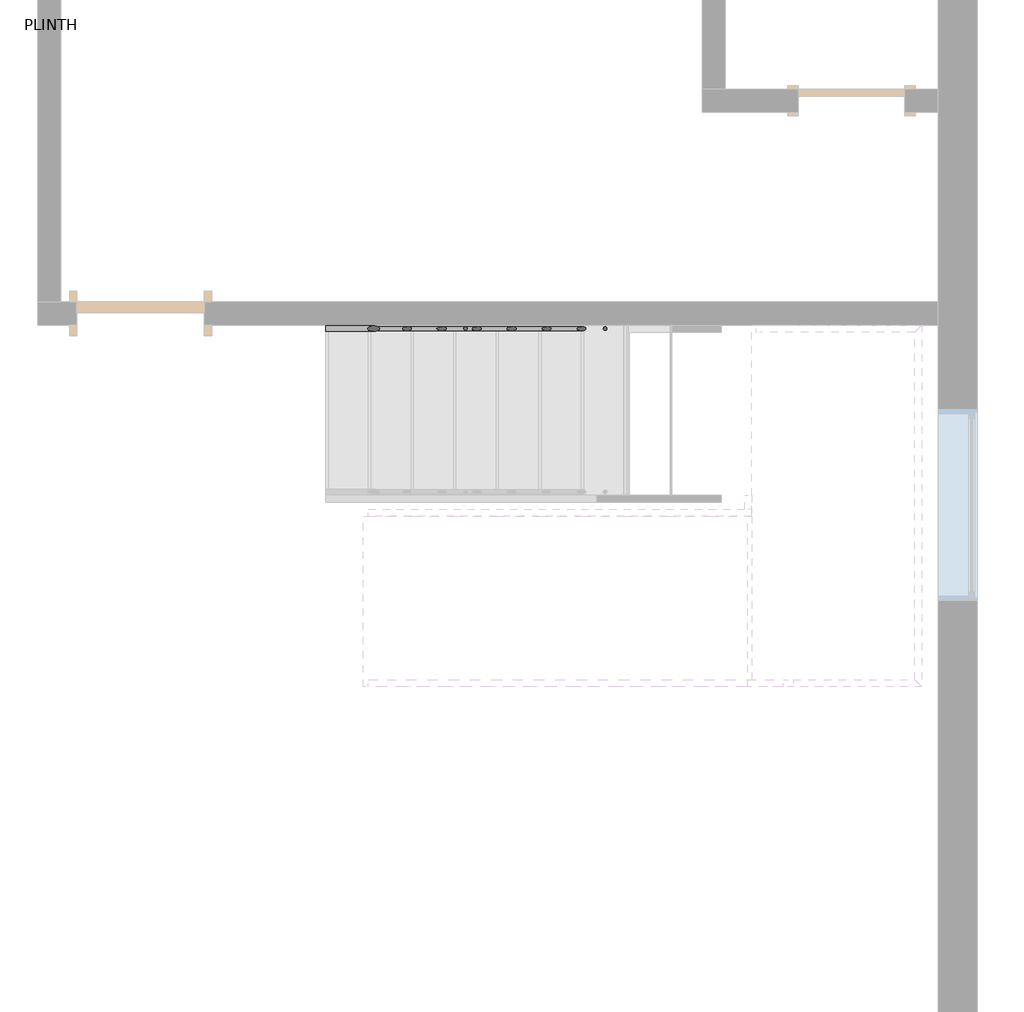
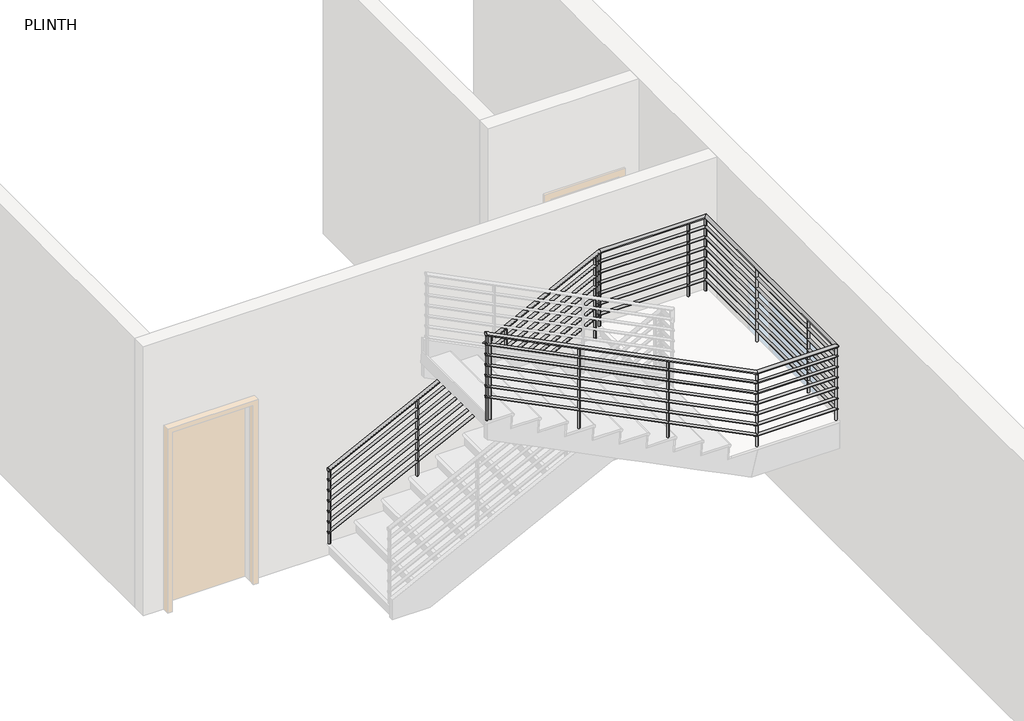
# One storey, part 3 of 4: 1 railing.
"""IFC4 building model written with IfcOpenShell, lengths in millimetres."""

from ifc_helpers import new_model, si_unit, point, frame, frame_2d, origin, place, context, project, spatial, circle_curve, ellipse_curve, trimmed, segment, composite_curve, outline, extrude, element, save
from ifc_brep_helpers import plane_surface, cylinder_surface, advanced_brep

model = new_model("IFC4")

# Units and contexts
model_context = context("Model", 3, world=origin())
ifc_project = project(units=[si_unit("LENGTHUNIT", "METRE", prefix="MILLI")], contexts=[model_context])

# Site, building, storey
site = spatial("IfcSite", under=ifc_project)
building = spatial("IfcBuilding", under=site)
storey = spatial("IfcBuildingStorey", under=building, Name="PLINTH", Elevation=0.0)

# Railing
placement = place(None, origin())
element("IfcRailing", 1, ObjectType="900mm Pipe", at=placement, inside=storey, context=model_context, shape_type="SolidModel", body=[
    advanced_brep(
    [(6849.4583908, 3581.0640673, 1030.0393202), (6849.4583908, 3621.0640673, 1030.0393202), (9902.1797503, 3581.0640673, 2556.4), (9902.1797503, 3621.0640673, 2556.4), (11071.2583908, 3581.0640673, 2556.4), (11111.2583908, 3621.0640673, 2556.4), (11071.2583908, 1083.4640673, 2556.4), (11111.2583908, 1043.4640673, 2556.4), (10197.5370312, 1083.4640673, 2556.4), (10197.5370312, 1043.4640673, 2556.4), (7154.2583908, 1083.4640673, 4078.0393202), (7154.2583908, 1043.4640673, 4078.0393202)],
    [
        (0, 1, ellipse_curve(frame((6849.4583908, 3601.0640673, 1030.0393202), z_axis=(-1.0, 0.0, 0.0), x_axis=(0.0, 0.0, -1.0)), 22.3606798, 20.0)),
        (1, 0, ellipse_curve(frame((6849.4583908, 3601.0640673, 1030.0393202), z_axis=(-1.0, 0.0, 0.0), x_axis=(0.0, 0.0, -1.0)), 22.3606798, 20.0)),
        (0, 2),
        (2, 3, ellipse_curve(frame((9902.1797503, 3601.0640673, 2556.4), z_axis=(-0.9732489894677303, 0.0, -0.22975292054736113), x_axis=(0.22975292054736202, 0.0, -0.97324898946773)), 20.5497259, 20.0)),
        (3, 1),
        (3, 2, ellipse_curve(frame((9902.1797503, 3601.0640673, 2556.4), z_axis=(-0.9732489894677303, 0.0, -0.22975292054736113), x_axis=(0.22975292054736202, 0.0, -0.97324898946773)), 20.5497259, 20.0)),
        (2, 4),
        (4, 5, ellipse_curve(frame((11091.2583908, 3601.0640673, 2556.4), z_axis=(-0.7071067811865462, 0.7071067811865488, 0.0), x_axis=(-0.7071067811865488, -0.7071067811865462, 0.0)), 28.2842712, 20.0)),
        (5, 3),
        (5, 4, ellipse_curve(frame((11091.2583908, 3601.0640673, 2556.4), z_axis=(-0.7071067811865462, 0.7071067811865488, 0.0), x_axis=(-0.7071067811865488, -0.7071067811865462, 0.0)), 28.2842712, 20.0)),
        (4, 6),
        (6, 7, ellipse_curve(frame((11091.2583908, 1063.4640673, 2556.4), z_axis=(0.7071067811865488, 0.7071067811865462, 0.0), x_axis=(-0.7071067811865462, 0.7071067811865488, 0.0)), 28.2842712, 20.0)),
        (7, 5),
        (7, 6, ellipse_curve(frame((11091.2583908, 1063.4640673, 2556.4), z_axis=(0.7071067811865488, 0.7071067811865462, 0.0), x_axis=(-0.7071067811865462, 0.7071067811865488, 0.0)), 28.2842712, 20.0)),
        (6, 8),
        (8, 9, ellipse_curve(frame((10197.5370312, 1063.4640673, 2556.4), z_axis=(0.9732489894677302, 0.0, -0.22975292054736135), x_axis=(0.22975292054736085, 0.0, 0.9732489894677303)), 20.5497259, 20.0)),
        (9, 7),
        (9, 8, ellipse_curve(frame((10197.5370312, 1063.4640673, 2556.4), z_axis=(0.9732489894677302, 0.0, -0.22975292054736135), x_axis=(0.22975292054736085, 0.0, 0.9732489894677303)), 20.5497259, 20.0)),
        (10, 11, ellipse_curve(frame((7154.2583908, 1063.4640673, 4078.0393202), z_axis=(-1.0, 0.0, 0.0), x_axis=(0.0, 0.0, -1.0)), 22.3606798, 20.0)),
        (11, 10, ellipse_curve(frame((7154.2583908, 1063.4640673, 4078.0393202), z_axis=(-1.0, 0.0, 0.0), x_axis=(0.0, 0.0, -1.0)), 22.3606798, 20.0)),
        (8, 10),
        (11, 9),
    ],
    [
        plane_surface(frame((6849.4583908, 3601.0640673, 1052.4), z_axis=(-1.0, 0.0, 0.0), x_axis=(0.0, 1.0, 0.0))),
        cylinder_surface(frame((6858.4026627, 3601.0640673, 1034.5114562), z_axis=(-0.894427190999916, 0.0, -0.4472135954999578), x_axis=(0.0, 1.0, 0.0)), 20.0),
        cylinder_surface(frame((9897.4583908, 3601.0640673, 2556.4), z_axis=(-1.0, 0.0, 0.0), x_axis=(0.0, 1.0, 0.0)), 20.0),
        cylinder_surface(frame((11091.2583908, 3601.0640673, 2556.4), z_axis=(0.0, 1.0, 0.0), x_axis=(1.0, 0.0, 0.0)), 20.0),
        cylinder_surface(frame((11091.2583908, 1063.4640673, 2556.4), z_axis=(1.0, 0.0, 0.0), x_axis=(0.0, -1.0, 0.0)), 20.0),
        plane_surface(frame((7154.2583908, 1063.4640673, 4100.4), z_axis=(-1.0, 0.0, 0.0), x_axis=(0.0, -1.0, 0.0))),
        cylinder_surface(frame((10193.3141188, 1063.4640673, 2558.5114562), z_axis=(0.8944271909999157, 0.0, -0.44721359549995826), x_axis=(0.0, -1.0, 0.0)), 20.0),
    ],
    [
        (0, [[1, 2]]),
        (1, [[-1, 3, 4, 5]]),
        (1, [[-2, -5, 6, -3]]),
        (2, [[-4, 7, 8, 9]]),
        (2, [[-6, -9, 10, -7]]),
        (3, [[-8, 11, 12, 13]]),
        (3, [[-10, -13, 14, -11]]),
        (4, [[-12, 15, 16, 17]]),
        (4, [[-14, -17, 18, -15]]),
        (5, [[19, 20]]),
        (6, [[-16, 21, -20, 22]]),
        (6, [[-18, -22, -19, -21]]),
    ],
),
    advanced_brep(
    [(6849.4583908, 3586.0640673, 910.6294902), (6849.4583908, 3616.0640673, 910.6294902), (9900.9994104, 3586.0640673, 2436.4), (9900.9994104, 3616.0640673, 2436.4), (11076.2583908, 3586.0640673, 2436.4), (11106.2583908, 3616.0640673, 2436.4), (11076.2583908, 1078.4640673, 2436.4), (11106.2583908, 1048.4640673, 2436.4), (10198.7173711, 1078.4640673, 2436.4), (10198.7173711, 1048.4640673, 2436.4), (7154.2583908, 1078.4640673, 3958.6294902), (7154.2583908, 1048.4640673, 3958.6294902)],
    [
        (0, 1, ellipse_curve(frame((6849.4583908, 3601.0640673, 910.6294902), z_axis=(-1.0, 0.0, 0.0), x_axis=(0.0, 0.0, -1.0)), 16.7705098, 15.0)),
        (1, 0, ellipse_curve(frame((6849.4583908, 3601.0640673, 910.6294902), z_axis=(-1.0, 0.0, 0.0), x_axis=(0.0, 0.0, -1.0)), 16.7705098, 15.0)),
        (0, 2),
        (2, 3, ellipse_curve(frame((9900.9994104, 3601.0640673, 2436.4), z_axis=(-0.9732489894677303, 0.0, -0.22975292054736116), x_axis=(0.22975292054736196, 0.0, -0.97324898946773)), 15.4122945, 15.0)),
        (3, 1),
        (3, 2, ellipse_curve(frame((9900.9994104, 3601.0640673, 2436.4), z_axis=(-0.9732489894677303, 0.0, -0.22975292054736116), x_axis=(0.22975292054736196, 0.0, -0.97324898946773)), 15.4122945, 15.0)),
        (2, 4),
        (4, 5, ellipse_curve(frame((11091.2583908, 3601.0640673, 2436.4), z_axis=(-0.7071067811865462, 0.7071067811865488, 0.0), x_axis=(-0.7071067811865488, -0.7071067811865462, 0.0)), 21.2132034, 15.0)),
        (5, 3),
        (5, 4, ellipse_curve(frame((11091.2583908, 3601.0640673, 2436.4), z_axis=(-0.7071067811865462, 0.7071067811865488, 0.0), x_axis=(-0.7071067811865488, -0.7071067811865462, 0.0)), 21.2132034, 15.0)),
        (4, 6),
        (6, 7, ellipse_curve(frame((11091.2583908, 1063.4640673, 2436.4), z_axis=(0.7071067811865488, 0.7071067811865462, 0.0), x_axis=(-0.7071067811865462, 0.7071067811865488, 0.0)), 21.2132034, 15.0)),
        (7, 5),
        (7, 6, ellipse_curve(frame((11091.2583908, 1063.4640673, 2436.4), z_axis=(0.7071067811865488, 0.7071067811865462, 0.0), x_axis=(-0.7071067811865462, 0.7071067811865488, 0.0)), 21.2132034, 15.0)),
        (6, 8),
        (8, 9, ellipse_curve(frame((10198.7173711, 1063.4640673, 2436.4), z_axis=(0.9732489894677302, 0.0, -0.22975292054736135), x_axis=(0.22975292054736085, 0.0, 0.9732489894677303)), 15.4122945, 15.0)),
        (9, 7),
        (9, 8, ellipse_curve(frame((10198.7173711, 1063.4640673, 2436.4), z_axis=(0.9732489894677302, 0.0, -0.22975292054736135), x_axis=(0.22975292054736085, 0.0, 0.9732489894677303)), 15.4122945, 15.0)),
        (10, 11, ellipse_curve(frame((7154.2583908, 1063.4640673, 3958.6294902), z_axis=(-1.0, 0.0, 0.0), x_axis=(0.0, 0.0, -1.0)), 16.7705098, 15.0)),
        (11, 10, ellipse_curve(frame((7154.2583908, 1063.4640673, 3958.6294902), z_axis=(-1.0, 0.0, 0.0), x_axis=(0.0, 0.0, -1.0)), 16.7705098, 15.0)),
        (8, 10),
        (11, 9),
    ],
    [
        plane_surface(frame((6849.4583908, 3601.0640673, 927.4), z_axis=(-1.0, 0.0, 0.0), x_axis=(0.0, 1.0, 0.0))),
        cylinder_surface(frame((6856.1665947, 3601.0640673, 913.9835921), z_axis=(-0.894427190999916, 0.0, -0.44721359549995787), x_axis=(0.0, 1.0, 0.0)), 15.0),
        cylinder_surface(frame((9897.4583908, 3601.0640673, 2436.4), z_axis=(-1.0, 0.0, 0.0), x_axis=(0.0, 1.0, 0.0)), 15.0),
        cylinder_surface(frame((11091.2583908, 3601.0640673, 2436.4), z_axis=(0.0, 1.0, 0.0), x_axis=(1.0, 0.0, 0.0)), 15.0),
        cylinder_surface(frame((11091.2583908, 1063.4640673, 2436.4), z_axis=(1.0, 0.0, 0.0), x_axis=(0.0, -1.0, 0.0)), 15.0),
        plane_surface(frame((7154.2583908, 1063.4640673, 3975.4), z_axis=(-1.0, 0.0, 0.0), x_axis=(0.0, -1.0, 0.0))),
        cylinder_surface(frame((10195.5501868, 1063.4640673, 2437.9835921), z_axis=(0.8944271909999157, 0.0, -0.44721359549995826), x_axis=(0.0, -1.0, 0.0)), 15.0),
    ],
    [
        (0, [[1, 2]]),
        (1, [[-1, 3, 4, 5]]),
        (1, [[-2, -5, 6, -3]]),
        (2, [[-4, 7, 8, 9]]),
        (2, [[-6, -9, 10, -7]]),
        (3, [[-8, 11, 12, 13]]),
        (3, [[-10, -13, 14, -11]]),
        (4, [[-12, 15, 16, 17]]),
        (4, [[-14, -17, 18, -15]]),
        (5, [[19, 20]]),
        (6, [[-16, 21, -20, 22]]),
        (6, [[-18, -22, -19, -21]]),
    ],
),
    advanced_brep(
    [(6849.4583908, 3586.0640673, 785.6294902), (6849.4583908, 3616.0640673, 785.6294902), (9900.9994104, 3586.0640673, 2311.4), (9900.9994104, 3616.0640673, 2311.4), (11076.2583908, 3586.0640673, 2311.4), (11106.2583908, 3616.0640673, 2311.4), (11076.2583908, 1078.4640673, 2311.4), (11106.2583908, 1048.4640673, 2311.4), (10198.7173711, 1078.4640673, 2311.4), (10198.7173711, 1048.4640673, 2311.4), (7154.2583908, 1078.4640673, 3833.6294902), (7154.2583908, 1048.4640673, 3833.6294902)],
    [
        (0, 1, ellipse_curve(frame((6849.4583908, 3601.0640673, 785.6294902), z_axis=(-1.0, 0.0, 0.0), x_axis=(0.0, 0.0, -1.0)), 16.7705098, 15.0)),
        (1, 0, ellipse_curve(frame((6849.4583908, 3601.0640673, 785.6294902), z_axis=(-1.0, 0.0, 0.0), x_axis=(0.0, 0.0, -1.0)), 16.7705098, 15.0)),
        (0, 2),
        (2, 3, ellipse_curve(frame((9900.9994104, 3601.0640673, 2311.4), z_axis=(-0.9732489894677303, 0.0, -0.22975292054736116), x_axis=(0.22975292054736196, 0.0, -0.97324898946773)), 15.4122945, 15.0)),
        (3, 1),
        (3, 2, ellipse_curve(frame((9900.9994104, 3601.0640673, 2311.4), z_axis=(-0.9732489894677303, 0.0, -0.22975292054736116), x_axis=(0.22975292054736196, 0.0, -0.97324898946773)), 15.4122945, 15.0)),
        (2, 4),
        (4, 5, ellipse_curve(frame((11091.2583908, 3601.0640673, 2311.4), z_axis=(-0.7071067811865462, 0.7071067811865488, 0.0), x_axis=(-0.7071067811865488, -0.7071067811865462, 0.0)), 21.2132034, 15.0)),
        (5, 3),
        (5, 4, ellipse_curve(frame((11091.2583908, 3601.0640673, 2311.4), z_axis=(-0.7071067811865462, 0.7071067811865488, 0.0), x_axis=(-0.7071067811865488, -0.7071067811865462, 0.0)), 21.2132034, 15.0)),
        (4, 6),
        (6, 7, ellipse_curve(frame((11091.2583908, 1063.4640673, 2311.4), z_axis=(0.7071067811865488, 0.7071067811865462, 0.0), x_axis=(-0.7071067811865462, 0.7071067811865488, 0.0)), 21.2132034, 15.0)),
        (7, 5),
        (7, 6, ellipse_curve(frame((11091.2583908, 1063.4640673, 2311.4), z_axis=(0.7071067811865488, 0.7071067811865462, 0.0), x_axis=(-0.7071067811865462, 0.7071067811865488, 0.0)), 21.2132034, 15.0)),
        (6, 8),
        (8, 9, ellipse_curve(frame((10198.7173711, 1063.4640673, 2311.4), z_axis=(0.9732489894677302, 0.0, -0.22975292054736132), x_axis=(0.22975292054736085, 0.0, 0.9732489894677302)), 15.4122945, 15.0)),
        (9, 7),
        (9, 8, ellipse_curve(frame((10198.7173711, 1063.4640673, 2311.4), z_axis=(0.9732489894677302, 0.0, -0.22975292054736132), x_axis=(0.22975292054736085, 0.0, 0.9732489894677302)), 15.4122945, 15.0)),
        (10, 11, ellipse_curve(frame((7154.2583908, 1063.4640673, 3833.6294902), z_axis=(-1.0, 0.0, 0.0), x_axis=(0.0, 0.0, -1.0)), 16.7705098, 15.0)),
        (11, 10, ellipse_curve(frame((7154.2583908, 1063.4640673, 3833.6294902), z_axis=(-1.0, 0.0, 0.0), x_axis=(0.0, 0.0, -1.0)), 16.7705098, 15.0)),
        (8, 10),
        (11, 9),
    ],
    [
        plane_surface(frame((6849.4583908, 3601.0640673, 802.4), z_axis=(-1.0, 0.0, 0.0), x_axis=(0.0, 1.0, 0.0))),
        cylinder_surface(frame((6856.1665947, 3601.0640673, 788.9835921), z_axis=(-0.894427190999916, 0.0, -0.44721359549995787), x_axis=(0.0, 1.0, 0.0)), 15.0),
        cylinder_surface(frame((9897.4583908, 3601.0640673, 2311.4), z_axis=(-1.0, 0.0, 0.0), x_axis=(0.0, 1.0, 0.0)), 15.0),
        cylinder_surface(frame((11091.2583908, 3601.0640673, 2311.4), z_axis=(0.0, 1.0, 0.0), x_axis=(1.0, 0.0, 0.0)), 15.0),
        cylinder_surface(frame((11091.2583908, 1063.4640673, 2311.4), z_axis=(1.0, 0.0, 0.0), x_axis=(0.0, -1.0, 0.0)), 15.0),
        plane_surface(frame((7154.2583908, 1063.4640673, 3850.4), z_axis=(-1.0, 0.0, 0.0), x_axis=(0.0, -1.0, 0.0))),
        cylinder_surface(frame((10195.5501868, 1063.4640673, 2312.9835921), z_axis=(0.8944271909999159, 0.0, -0.4472135954999582), x_axis=(0.0, -1.0, 0.0)), 15.0),
    ],
    [
        (0, [[1, 2]]),
        (1, [[-1, 3, 4, 5]]),
        (1, [[-2, -5, 6, -3]]),
        (2, [[-4, 7, 8, 9]]),
        (2, [[-6, -9, 10, -7]]),
        (3, [[-8, 11, 12, 13]]),
        (3, [[-10, -13, 14, -11]]),
        (4, [[-12, 15, 16, 17]]),
        (4, [[-14, -17, 18, -15]]),
        (5, [[19, 20]]),
        (6, [[-16, 21, -20, 22]]),
        (6, [[-18, -22, -19, -21]]),
    ],
),
    advanced_brep(
    [(6849.4583908, 3586.0640673, 660.6294902), (6849.4583908, 3616.0640673, 660.6294902), (9900.9994104, 3586.0640673, 2186.4), (9900.9994104, 3616.0640673, 2186.4), (11076.2583908, 3586.0640673, 2186.4), (11106.2583908, 3616.0640673, 2186.4), (11076.2583908, 1078.4640673, 2186.4), (11106.2583908, 1048.4640673, 2186.4), (10198.7173711, 1078.4640673, 2186.4), (10198.7173711, 1048.4640673, 2186.4), (7154.2583908, 1078.4640673, 3708.6294902), (7154.2583908, 1048.4640673, 3708.6294902)],
    [
        (0, 1, ellipse_curve(frame((6849.4583908, 3601.0640673, 660.6294902), z_axis=(-1.0, 0.0, 0.0), x_axis=(0.0, 0.0, -1.0)), 16.7705098, 15.0)),
        (1, 0, ellipse_curve(frame((6849.4583908, 3601.0640673, 660.6294902), z_axis=(-1.0, 0.0, 0.0), x_axis=(0.0, 0.0, -1.0)), 16.7705098, 15.0)),
        (0, 2),
        (2, 3, ellipse_curve(frame((9900.9994104, 3601.0640673, 2186.4), z_axis=(-0.9732489894677303, 0.0, -0.22975292054736116), x_axis=(0.22975292054736196, 0.0, -0.97324898946773)), 15.4122945, 15.0)),
        (3, 1),
        (3, 2, ellipse_curve(frame((9900.9994104, 3601.0640673, 2186.4), z_axis=(-0.9732489894677303, 0.0, -0.22975292054736116), x_axis=(0.22975292054736196, 0.0, -0.97324898946773)), 15.4122945, 15.0)),
        (2, 4),
        (4, 5, ellipse_curve(frame((11091.2583908, 3601.0640673, 2186.4), z_axis=(-0.7071067811865462, 0.7071067811865488, 0.0), x_axis=(-0.7071067811865488, -0.7071067811865462, 0.0)), 21.2132034, 15.0)),
        (5, 3),
        (5, 4, ellipse_curve(frame((11091.2583908, 3601.0640673, 2186.4), z_axis=(-0.7071067811865462, 0.7071067811865488, 0.0), x_axis=(-0.7071067811865488, -0.7071067811865462, 0.0)), 21.2132034, 15.0)),
        (4, 6),
        (6, 7, ellipse_curve(frame((11091.2583908, 1063.4640673, 2186.4), z_axis=(0.7071067811865488, 0.7071067811865462, 0.0), x_axis=(-0.7071067811865462, 0.7071067811865488, 0.0)), 21.2132034, 15.0)),
        (7, 5),
        (7, 6, ellipse_curve(frame((11091.2583908, 1063.4640673, 2186.4), z_axis=(0.7071067811865488, 0.7071067811865462, 0.0), x_axis=(-0.7071067811865462, 0.7071067811865488, 0.0)), 21.2132034, 15.0)),
        (6, 8),
        (8, 9, ellipse_curve(frame((10198.7173711, 1063.4640673, 2186.4), z_axis=(0.9732489894677302, 0.0, -0.22975292054736132), x_axis=(0.22975292054736085, 0.0, 0.9732489894677302)), 15.4122945, 15.0)),
        (9, 7),
        (9, 8, ellipse_curve(frame((10198.7173711, 1063.4640673, 2186.4), z_axis=(0.9732489894677302, 0.0, -0.22975292054736132), x_axis=(0.22975292054736085, 0.0, 0.9732489894677302)), 15.4122945, 15.0)),
        (10, 11, ellipse_curve(frame((7154.2583908, 1063.4640673, 3708.6294902), z_axis=(-1.0, 0.0, 0.0), x_axis=(0.0, 0.0, -1.0)), 16.7705098, 15.0)),
        (11, 10, ellipse_curve(frame((7154.2583908, 1063.4640673, 3708.6294902), z_axis=(-1.0, 0.0, 0.0), x_axis=(0.0, 0.0, -1.0)), 16.7705098, 15.0)),
        (8, 10),
        (11, 9),
    ],
    [
        plane_surface(frame((6849.4583908, 3601.0640673, 677.4), z_axis=(-1.0, 0.0, 0.0), x_axis=(0.0, 1.0, 0.0))),
        cylinder_surface(frame((6856.1665947, 3601.0640673, 663.9835921), z_axis=(-0.894427190999916, 0.0, -0.44721359549995787), x_axis=(0.0, 1.0, 0.0)), 15.0),
        cylinder_surface(frame((9897.4583908, 3601.0640673, 2186.4), z_axis=(-1.0, 0.0, 0.0), x_axis=(0.0, 1.0, 0.0)), 15.0),
        cylinder_surface(frame((11091.2583908, 3601.0640673, 2186.4), z_axis=(0.0, 1.0, 0.0), x_axis=(1.0, 0.0, 0.0)), 15.0),
        cylinder_surface(frame((11091.2583908, 1063.4640673, 2186.4), z_axis=(1.0, 0.0, 0.0), x_axis=(0.0, -1.0, 0.0)), 15.0),
        plane_surface(frame((7154.2583908, 1063.4640673, 3725.4), z_axis=(-1.0, 0.0, 0.0), x_axis=(0.0, -1.0, 0.0))),
        cylinder_surface(frame((10195.5501868, 1063.4640673, 2187.9835921), z_axis=(0.8944271909999159, 0.0, -0.4472135954999582), x_axis=(0.0, -1.0, 0.0)), 15.0),
    ],
    [
        (0, [[1, 2]]),
        (1, [[-1, 3, 4, 5]]),
        (1, [[-2, -5, 6, -3]]),
        (2, [[-4, 7, 8, 9]]),
        (2, [[-6, -9, 10, -7]]),
        (3, [[-8, 11, 12, 13]]),
        (3, [[-10, -13, 14, -11]]),
        (4, [[-12, 15, 16, 17]]),
        (4, [[-14, -17, 18, -15]]),
        (5, [[19, 20]]),
        (6, [[-16, 21, -20, 22]]),
        (6, [[-18, -22, -19, -21]]),
    ],
),
    advanced_brep(
    [(6849.4583908, 3586.0640673, 535.6294902), (6849.4583908, 3616.0640673, 535.6294902), (9900.9994104, 3586.0640673, 2061.4), (9900.9994104, 3616.0640673, 2061.4), (11076.2583908, 3586.0640673, 2061.4), (11106.2583908, 3616.0640673, 2061.4), (11076.2583908, 1078.4640673, 2061.4), (11106.2583908, 1048.4640673, 2061.4), (10198.7173711, 1078.4640673, 2061.4), (10198.7173711, 1048.4640673, 2061.4), (7154.2583908, 1078.4640673, 3583.6294902), (7154.2583908, 1048.4640673, 3583.6294902)],
    [
        (0, 1, ellipse_curve(frame((6849.4583908, 3601.0640673, 535.6294902), z_axis=(-1.0, 0.0, 0.0), x_axis=(0.0, 0.0, -1.0)), 16.7705098, 15.0)),
        (1, 0, ellipse_curve(frame((6849.4583908, 3601.0640673, 535.6294902), z_axis=(-1.0, 0.0, 0.0), x_axis=(0.0, 0.0, -1.0)), 16.7705098, 15.0)),
        (0, 2),
        (2, 3, ellipse_curve(frame((9900.9994104, 3601.0640673, 2061.4), z_axis=(-0.9732489894677303, 0.0, -0.22975292054736116), x_axis=(0.22975292054736196, 0.0, -0.97324898946773)), 15.4122945, 15.0)),
        (3, 1),
        (3, 2, ellipse_curve(frame((9900.9994104, 3601.0640673, 2061.4), z_axis=(-0.9732489894677303, 0.0, -0.22975292054736116), x_axis=(0.22975292054736196, 0.0, -0.97324898946773)), 15.4122945, 15.0)),
        (2, 4),
        (4, 5, ellipse_curve(frame((11091.2583908, 3601.0640673, 2061.4), z_axis=(-0.7071067811865462, 0.7071067811865488, 0.0), x_axis=(-0.7071067811865488, -0.7071067811865462, 0.0)), 21.2132034, 15.0)),
        (5, 3),
        (5, 4, ellipse_curve(frame((11091.2583908, 3601.0640673, 2061.4), z_axis=(-0.7071067811865462, 0.7071067811865488, 0.0), x_axis=(-0.7071067811865488, -0.7071067811865462, 0.0)), 21.2132034, 15.0)),
        (4, 6),
        (6, 7, ellipse_curve(frame((11091.2583908, 1063.4640673, 2061.4), z_axis=(0.7071067811865488, 0.7071067811865462, 0.0), x_axis=(-0.7071067811865462, 0.7071067811865488, 0.0)), 21.2132034, 15.0)),
        (7, 5),
        (7, 6, ellipse_curve(frame((11091.2583908, 1063.4640673, 2061.4), z_axis=(0.7071067811865488, 0.7071067811865462, 0.0), x_axis=(-0.7071067811865462, 0.7071067811865488, 0.0)), 21.2132034, 15.0)),
        (6, 8),
        (8, 9, ellipse_curve(frame((10198.7173711, 1063.4640673, 2061.4), z_axis=(0.9732489894677302, 0.0, -0.22975292054736132), x_axis=(0.22975292054736085, 0.0, 0.9732489894677302)), 15.4122945, 15.0)),
        (9, 7),
        (9, 8, ellipse_curve(frame((10198.7173711, 1063.4640673, 2061.4), z_axis=(0.9732489894677302, 0.0, -0.22975292054736132), x_axis=(0.22975292054736085, 0.0, 0.9732489894677302)), 15.4122945, 15.0)),
        (10, 11, ellipse_curve(frame((7154.2583908, 1063.4640673, 3583.6294902), z_axis=(-1.0, 0.0, 0.0), x_axis=(0.0, 0.0, -1.0)), 16.7705098, 15.0)),
        (11, 10, ellipse_curve(frame((7154.2583908, 1063.4640673, 3583.6294902), z_axis=(-1.0, 0.0, 0.0), x_axis=(0.0, 0.0, -1.0)), 16.7705098, 15.0)),
        (8, 10),
        (11, 9),
    ],
    [
        plane_surface(frame((6849.4583908, 3601.0640673, 552.4), z_axis=(-1.0, 0.0, 0.0), x_axis=(0.0, 1.0, 0.0))),
        cylinder_surface(frame((6856.1665947, 3601.0640673, 538.9835921), z_axis=(-0.894427190999916, 0.0, -0.44721359549995787), x_axis=(0.0, 1.0, 0.0)), 15.0),
        cylinder_surface(frame((9897.4583908, 3601.0640673, 2061.4), z_axis=(-1.0, 0.0, 0.0), x_axis=(0.0, 1.0, 0.0)), 15.0),
        cylinder_surface(frame((11091.2583908, 3601.0640673, 2061.4), z_axis=(0.0, 1.0, 0.0), x_axis=(1.0, 0.0, 0.0)), 15.0),
        cylinder_surface(frame((11091.2583908, 1063.4640673, 2061.4), z_axis=(1.0, 0.0, 0.0), x_axis=(0.0, -1.0, 0.0)), 15.0),
        plane_surface(frame((7154.2583908, 1063.4640673, 3600.4), z_axis=(-1.0, 0.0, 0.0), x_axis=(0.0, -1.0, 0.0))),
        cylinder_surface(frame((10195.5501868, 1063.4640673, 2062.9835921), z_axis=(0.8944271909999159, 0.0, -0.4472135954999582), x_axis=(0.0, -1.0, 0.0)), 15.0),
    ],
    [
        (0, [[1, 2]]),
        (1, [[-1, 3, 4, 5]]),
        (1, [[-2, -5, 6, -3]]),
        (2, [[-4, 7, 8, 9]]),
        (2, [[-6, -9, 10, -7]]),
        (3, [[-8, 11, 12, 13]]),
        (3, [[-10, -13, 14, -11]]),
        (4, [[-12, 15, 16, 17]]),
        (4, [[-14, -17, 18, -15]]),
        (5, [[19, 20]]),
        (6, [[-16, 21, -20, 22]]),
        (6, [[-18, -22, -19, -21]]),
    ],
),
    advanced_brep(
    [(6849.4583908, 3586.0640673, 410.6294902), (6849.4583908, 3616.0640673, 410.6294902), (9900.9994104, 3586.0640673, 1936.4), (9900.9994104, 3616.0640673, 1936.4), (11076.2583908, 3586.0640673, 1936.4), (11106.2583908, 3616.0640673, 1936.4), (11076.2583908, 1078.4640673, 1936.4), (11106.2583908, 1048.4640673, 1936.4), (10198.7173711, 1078.4640673, 1936.4), (10198.7173711, 1048.4640673, 1936.4), (7154.2583908, 1078.4640673, 3458.6294902), (7154.2583908, 1048.4640673, 3458.6294902)],
    [
        (0, 1, ellipse_curve(frame((6849.4583908, 3601.0640673, 410.6294902), z_axis=(-1.0, 0.0, 0.0), x_axis=(0.0, 0.0, -1.0)), 16.7705098, 15.0)),
        (1, 0, ellipse_curve(frame((6849.4583908, 3601.0640673, 410.6294902), z_axis=(-1.0, 0.0, 0.0), x_axis=(0.0, 0.0, -1.0)), 16.7705098, 15.0)),
        (0, 2),
        (2, 3, ellipse_curve(frame((9900.9994104, 3601.0640673, 1936.4), z_axis=(-0.9732489894677303, 0.0, -0.22975292054736116), x_axis=(0.22975292054736196, 0.0, -0.97324898946773)), 15.4122945, 15.0)),
        (3, 1),
        (3, 2, ellipse_curve(frame((9900.9994104, 3601.0640673, 1936.4), z_axis=(-0.9732489894677303, 0.0, -0.22975292054736116), x_axis=(0.22975292054736196, 0.0, -0.97324898946773)), 15.4122945, 15.0)),
        (2, 4),
        (4, 5, ellipse_curve(frame((11091.2583908, 3601.0640673, 1936.4), z_axis=(-0.7071067811865462, 0.7071067811865488, 0.0), x_axis=(-0.7071067811865488, -0.7071067811865462, 0.0)), 21.2132034, 15.0)),
        (5, 3),
        (5, 4, ellipse_curve(frame((11091.2583908, 3601.0640673, 1936.4), z_axis=(-0.7071067811865462, 0.7071067811865488, 0.0), x_axis=(-0.7071067811865488, -0.7071067811865462, 0.0)), 21.2132034, 15.0)),
        (4, 6),
        (6, 7, ellipse_curve(frame((11091.2583908, 1063.4640673, 1936.4), z_axis=(0.7071067811865488, 0.7071067811865462, 0.0), x_axis=(-0.7071067811865462, 0.7071067811865488, 0.0)), 21.2132034, 15.0)),
        (7, 5),
        (7, 6, ellipse_curve(frame((11091.2583908, 1063.4640673, 1936.4), z_axis=(0.7071067811865488, 0.7071067811865462, 0.0), x_axis=(-0.7071067811865462, 0.7071067811865488, 0.0)), 21.2132034, 15.0)),
        (6, 8),
        (8, 9, ellipse_curve(frame((10198.7173711, 1063.4640673, 1936.4), z_axis=(0.9732489894677302, 0.0, -0.22975292054736135), x_axis=(0.22975292054736085, 0.0, 0.9732489894677303)), 15.4122945, 15.0)),
        (9, 7),
        (9, 8, ellipse_curve(frame((10198.7173711, 1063.4640673, 1936.4), z_axis=(0.9732489894677302, 0.0, -0.22975292054736135), x_axis=(0.22975292054736085, 0.0, 0.9732489894677303)), 15.4122945, 15.0)),
        (10, 11, ellipse_curve(frame((7154.2583908, 1063.4640673, 3458.6294902), z_axis=(-1.0, 0.0, 0.0), x_axis=(0.0, 0.0, -1.0)), 16.7705098, 15.0)),
        (11, 10, ellipse_curve(frame((7154.2583908, 1063.4640673, 3458.6294902), z_axis=(-1.0, 0.0, 0.0), x_axis=(0.0, 0.0, -1.0)), 16.7705098, 15.0)),
        (8, 10),
        (11, 9),
    ],
    [
        plane_surface(frame((6849.4583908, 3601.0640673, 427.4), z_axis=(-1.0, 0.0, 0.0), x_axis=(0.0, 1.0, 0.0))),
        cylinder_surface(frame((6856.1665947, 3601.0640673, 413.9835921), z_axis=(-0.894427190999916, 0.0, -0.44721359549995787), x_axis=(0.0, 1.0, 0.0)), 15.0),
        cylinder_surface(frame((9897.4583908, 3601.0640673, 1936.4), z_axis=(-1.0, 0.0, 0.0), x_axis=(0.0, 1.0, 0.0)), 15.0),
        cylinder_surface(frame((11091.2583908, 3601.0640673, 1936.4), z_axis=(0.0, 1.0, 0.0), x_axis=(1.0, 0.0, 0.0)), 15.0),
        cylinder_surface(frame((11091.2583908, 1063.4640673, 1936.4), z_axis=(1.0, 0.0, 0.0), x_axis=(0.0, -1.0, 0.0)), 15.0),
        plane_surface(frame((7154.2583908, 1063.4640673, 3475.4), z_axis=(-1.0, 0.0, 0.0), x_axis=(0.0, -1.0, 0.0))),
        cylinder_surface(frame((10195.5501868, 1063.4640673, 1937.9835921), z_axis=(0.8944271909999157, 0.0, -0.44721359549995826), x_axis=(0.0, -1.0, 0.0)), 15.0),
    ],
    [
        (0, [[1, 2]]),
        (1, [[-1, 3, 4, 5]]),
        (1, [[-2, -5, 6, -3]]),
        (2, [[-4, 7, 8, 9]]),
        (2, [[-6, -9, 10, -7]]),
        (3, [[-8, 11, 12, 13]]),
        (3, [[-10, -13, 14, -11]]),
        (4, [[-12, 15, 16, 17]]),
        (4, [[-14, -17, 18, -15]]),
        (5, [[19, 20]]),
        (6, [[-16, 21, -20, 22]]),
        (6, [[-18, -22, -19, -21]]),
    ],
),
    advanced_brep(
    [(6849.4583908, 3586.0640673, 285.6294902), (6849.4583908, 3616.0640673, 285.6294902), (9900.9994104, 3586.0640673, 1811.4), (9900.9994104, 3616.0640673, 1811.4), (11076.2583908, 3586.0640673, 1811.4), (11106.2583908, 3616.0640673, 1811.4), (11076.2583908, 1078.4640673, 1811.4), (11106.2583908, 1048.4640673, 1811.4), (10198.7173711, 1078.4640673, 1811.4), (10198.7173711, 1048.4640673, 1811.4), (7154.2583908, 1078.4640673, 3333.6294902), (7154.2583908, 1048.4640673, 3333.6294902)],
    [
        (0, 1, ellipse_curve(frame((6849.4583908, 3601.0640673, 285.6294902), z_axis=(-1.0, 0.0, 0.0), x_axis=(0.0, 0.0, -1.0)), 16.7705098, 15.0)),
        (1, 0, ellipse_curve(frame((6849.4583908, 3601.0640673, 285.6294902), z_axis=(-1.0, 0.0, 0.0), x_axis=(0.0, 0.0, -1.0)), 16.7705098, 15.0)),
        (0, 2),
        (2, 3, ellipse_curve(frame((9900.9994104, 3601.0640673, 1811.4), z_axis=(-0.9732489894677303, 0.0, -0.22975292054736116), x_axis=(0.22975292054736196, 0.0, -0.97324898946773)), 15.4122945, 15.0)),
        (3, 1),
        (3, 2, ellipse_curve(frame((9900.9994104, 3601.0640673, 1811.4), z_axis=(-0.9732489894677303, 0.0, -0.22975292054736116), x_axis=(0.22975292054736196, 0.0, -0.97324898946773)), 15.4122945, 15.0)),
        (2, 4),
        (4, 5, ellipse_curve(frame((11091.2583908, 3601.0640673, 1811.4), z_axis=(-0.7071067811865462, 0.7071067811865488, 0.0), x_axis=(-0.7071067811865488, -0.7071067811865462, 0.0)), 21.2132034, 15.0)),
        (5, 3),
        (5, 4, ellipse_curve(frame((11091.2583908, 3601.0640673, 1811.4), z_axis=(-0.7071067811865462, 0.7071067811865488, 0.0), x_axis=(-0.7071067811865488, -0.7071067811865462, 0.0)), 21.2132034, 15.0)),
        (4, 6),
        (6, 7, ellipse_curve(frame((11091.2583908, 1063.4640673, 1811.4), z_axis=(0.7071067811865488, 0.7071067811865462, 0.0), x_axis=(-0.7071067811865462, 0.7071067811865488, 0.0)), 21.2132034, 15.0)),
        (7, 5),
        (7, 6, ellipse_curve(frame((11091.2583908, 1063.4640673, 1811.4), z_axis=(0.7071067811865488, 0.7071067811865462, 0.0), x_axis=(-0.7071067811865462, 0.7071067811865488, 0.0)), 21.2132034, 15.0)),
        (6, 8),
        (8, 9, ellipse_curve(frame((10198.7173711, 1063.4640673, 1811.4), z_axis=(0.9732489894677302, 0.0, -0.22975292054736132), x_axis=(0.22975292054736085, 0.0, 0.9732489894677302)), 15.4122945, 15.0)),
        (9, 7),
        (9, 8, ellipse_curve(frame((10198.7173711, 1063.4640673, 1811.4), z_axis=(0.9732489894677302, 0.0, -0.22975292054736132), x_axis=(0.22975292054736085, 0.0, 0.9732489894677302)), 15.4122945, 15.0)),
        (10, 11, ellipse_curve(frame((7154.2583908, 1063.4640673, 3333.6294902), z_axis=(-1.0, 0.0, 0.0), x_axis=(0.0, 0.0, -1.0)), 16.7705098, 15.0)),
        (11, 10, ellipse_curve(frame((7154.2583908, 1063.4640673, 3333.6294902), z_axis=(-1.0, 0.0, 0.0), x_axis=(0.0, 0.0, -1.0)), 16.7705098, 15.0)),
        (8, 10),
        (11, 9),
    ],
    [
        plane_surface(frame((6849.4583908, 3601.0640673, 302.4), z_axis=(-1.0, 0.0, 0.0), x_axis=(0.0, 1.0, 0.0))),
        cylinder_surface(frame((6856.1665947, 3601.0640673, 288.9835921), z_axis=(-0.894427190999916, 0.0, -0.44721359549995787), x_axis=(0.0, 1.0, 0.0)), 15.0),
        cylinder_surface(frame((9897.4583908, 3601.0640673, 1811.4), z_axis=(-1.0, 0.0, 0.0), x_axis=(0.0, 1.0, 0.0)), 15.0),
        cylinder_surface(frame((11091.2583908, 3601.0640673, 1811.4), z_axis=(0.0, 1.0, 0.0), x_axis=(1.0, 0.0, 0.0)), 15.0),
        cylinder_surface(frame((11091.2583908, 1063.4640673, 1811.4), z_axis=(1.0, 0.0, 0.0), x_axis=(0.0, -1.0, 0.0)), 15.0),
        plane_surface(frame((7154.2583908, 1063.4640673, 3350.4), z_axis=(-1.0, 0.0, 0.0), x_axis=(0.0, -1.0, 0.0))),
        cylinder_surface(frame((10195.5501868, 1063.4640673, 1812.9835921), z_axis=(0.8944271909999159, 0.0, -0.4472135954999582), x_axis=(0.0, -1.0, 0.0)), 15.0),
    ],
    [
        (0, [[1, 2]]),
        (1, [[-1, 3, 4, 5]]),
        (1, [[-2, -5, 6, -3]]),
        (2, [[-4, 7, 8, 9]]),
        (2, [[-6, -9, 10, -7]]),
        (3, [[-8, 11, 12, 13]]),
        (3, [[-10, -13, 14, -11]]),
        (4, [[-12, 15, 16, 17]]),
        (4, [[-14, -17, 18, -15]]),
        (5, [[19, 20]]),
        (6, [[-16, 21, -20, 22]]),
        (6, [[-18, -22, -19, -21]]),
    ],
),
    advanced_brep(
    [(7202.2583908, 1050.9640673, 4031.6786405), (7202.2583908, 1075.9640673, 4031.6786405), (7202.2583908, 1075.9640673, 3048.0), (7202.2583908, 1050.9640673, 3048.0)],
    [
        (0, 1, ellipse_curve(frame((7202.2583908, 1063.4640673, 4031.6786405), z_axis=(-0.447213595499958, 0.0, -0.894427190999916), x_axis=(-0.8944271909999161, 0.0, 0.4472135954999576)), 13.9754249, 12.5)),
        (1, 2),
        (2, 3, circle_curve(frame((7202.2583908, 1063.4640673, 3048.0), z_axis=(0.0, 0.0, 1.0), x_axis=(0.0, 1.0, 0.0)), 12.5)),
        (3, 0),
        (3, 2, circle_curve(frame((7202.2583908, 1063.4640673, 3048.0), z_axis=(0.0, 0.0, 1.0), x_axis=(0.0, 1.0, 0.0)), 12.5)),
        (1, 0, ellipse_curve(frame((7202.2583908, 1063.4640673, 4031.6786405), z_axis=(-0.447213595499958, 0.0, -0.894427190999916), x_axis=(-0.8944271909999161, 0.0, 0.4472135954999576)), 13.9754249, 12.5)),
    ],
    [
        cylinder_surface(frame((7202.2583908, 1063.4640673, 2948.0), z_axis=(0.0, 0.0, 1.0), x_axis=(0.0, 1.0, 0.0)), 12.5),
        plane_surface(frame((7177.2583908, 1088.4640673, 4044.1786405), z_axis=(0.447213595499958, 0.0, 0.894427190999916), x_axis=(0.0, -1.0, 0.0))),
        plane_surface(frame((7227.2583908, 1088.4640673, 3048.0), z_axis=(0.0, 0.0, -1.0), x_axis=(0.0, -1.0, 0.0))),
    ],
    [
        (0, [[1, 2, 3, 4]]),
        (0, [[5, -2, 6, -4]]),
        (1, [[-6, -1]]),
        (2, [[-5, -3]]),
    ],
),
    advanced_brep(
    [(8202.2583908, 1050.9640673, 3531.6786405), (8202.2583908, 1075.9640673, 3531.6786405), (8202.2583908, 1075.9640673, 2590.8), (8202.2583908, 1050.9640673, 2590.8)],
    [
        (0, 1, ellipse_curve(frame((8202.2583908, 1063.4640673, 3531.6786405), z_axis=(-0.447213595499958, 0.0, -0.894427190999916), x_axis=(-0.8944271909999161, 0.0, 0.4472135954999576)), 13.9754249, 12.5)),
        (1, 2),
        (2, 3, circle_curve(frame((8202.2583908, 1063.4640673, 2590.8), z_axis=(0.0, 0.0, 1.0), x_axis=(0.0, 1.0, 0.0)), 12.5)),
        (3, 0),
        (3, 2, circle_curve(frame((8202.2583908, 1063.4640673, 2590.8), z_axis=(0.0, 0.0, 1.0), x_axis=(0.0, 1.0, 0.0)), 12.5)),
        (1, 0, ellipse_curve(frame((8202.2583908, 1063.4640673, 3531.6786405), z_axis=(-0.447213595499958, 0.0, -0.894427190999916), x_axis=(-0.8944271909999161, 0.0, 0.4472135954999576)), 13.9754249, 12.5)),
    ],
    [
        cylinder_surface(frame((8202.2583908, 1063.4640673, 2490.8), z_axis=(0.0, 0.0, 1.0), x_axis=(0.0, 1.0, 0.0)), 12.5),
        plane_surface(frame((8177.2583908, 1088.4640673, 3544.1786405), z_axis=(0.447213595499958, 0.0, 0.894427190999916), x_axis=(0.0, -1.0, 0.0))),
        plane_surface(frame((8227.2583908, 1088.4640673, 2590.8), z_axis=(0.0, 0.0, -1.0), x_axis=(0.0, -1.0, 0.0))),
    ],
    [
        (0, [[1, 2, 3, 4]]),
        (0, [[5, -2, 6, -4]]),
        (1, [[-6, -1]]),
        (2, [[-5, -3]]),
    ],
),
    advanced_brep(
    [(9202.2583908, 1050.9640673, 3031.6786405), (9202.2583908, 1075.9640673, 3031.6786405), (9202.2583908, 1075.9640673, 2133.6), (9202.2583908, 1050.9640673, 2133.6)],
    [
        (0, 1, ellipse_curve(frame((9202.2583908, 1063.4640673, 3031.6786405), z_axis=(-0.44721359549995604, 0.0, -0.894427190999917), x_axis=(-0.8944271909999172, 0.0, 0.4472135954999556)), 13.9754249, 12.5)),
        (1, 2),
        (2, 3, circle_curve(frame((9202.2583908, 1063.4640673, 2133.6), z_axis=(0.0, 0.0, 1.0), x_axis=(0.0, 1.0, 0.0)), 12.5)),
        (3, 0),
        (3, 2, circle_curve(frame((9202.2583908, 1063.4640673, 2133.6), z_axis=(0.0, 0.0, 1.0), x_axis=(0.0, 1.0, 0.0)), 12.5)),
        (1, 0, ellipse_curve(frame((9202.2583908, 1063.4640673, 3031.6786405), z_axis=(-0.44721359549995604, 0.0, -0.894427190999917), x_axis=(-0.8944271909999172, 0.0, 0.4472135954999556)), 13.9754249, 12.5)),
    ],
    [
        cylinder_surface(frame((9202.2583908, 1063.4640673, 2033.6), z_axis=(0.0, 0.0, 1.0), x_axis=(0.0, 1.0, 0.0)), 12.5),
        plane_surface(frame((9177.2583908, 1088.4640673, 3044.1786405), z_axis=(0.44721359549995604, 0.0, 0.894427190999917), x_axis=(0.0, -1.0, 0.0))),
        plane_surface(frame((9227.2583908, 1088.4640673, 2133.6), z_axis=(0.0, 0.0, -1.0), x_axis=(0.0, -1.0, 0.0))),
    ],
    [
        (0, [[1, 2, 3, 4]]),
        (0, [[5, -2, 6, -4]]),
        (1, [[-6, -1]]),
        (2, [[-5, -3]]),
    ],
),
    extrude(outline(composite_curve([segment(trimmed(circle_curve(frame_2d((11091.2583908, 1601.0640673)), 12.5), [point((11078.7583908, 1601.0640673))], [point((11103.7583908, 1601.0640673))], False, "CARTESIAN"), True, "CONTINUOUS"), segment(trimmed(circle_curve(frame_2d((11091.2583908, 1601.0640673)), 12.5), [point((11103.7583908, 1601.0640673))], [point((11078.7583908, 1601.0640673))], False, "CARTESIAN"), True, "CONTINUOUS")], self_intersect=False)), frame((0.0, 0.0, 1676.4), z_axis=(0.0, 0.0, 1.0), x_axis=(1.0, 0.0, 0.0)), (0.0, 0.0, 1.0), 860.0),
    extrude(outline(composite_curve([segment(trimmed(circle_curve(frame_2d((11091.2583908, 2601.0640673)), 12.5), [point((11078.7583908, 2601.0640673))], [point((11103.7583908, 2601.0640673))], False, "CARTESIAN"), True, "CONTINUOUS"), segment(trimmed(circle_curve(frame_2d((11091.2583908, 2601.0640673)), 12.5), [point((11103.7583908, 2601.0640673))], [point((11078.7583908, 2601.0640673))], False, "CARTESIAN"), True, "CONTINUOUS")], self_intersect=False)), frame((0.0, 0.0, 1676.4), z_axis=(0.0, 0.0, 1.0), x_axis=(1.0, 0.0, 0.0)), (0.0, 0.0, 1.0), 860.0),
    extrude(outline(composite_curve([segment(trimmed(circle_curve(frame_2d((10897.4583908, 3601.0640673)), 12.5), [point((10897.4583908, 3588.5640673))], [point((10897.4583908, 3613.5640673))], False, "CARTESIAN"), True, "CONTINUOUS"), segment(trimmed(circle_curve(frame_2d((10897.4583908, 3601.0640673)), 12.5), [point((10897.4583908, 3613.5640673))], [point((10897.4583908, 3588.5640673))], False, "CARTESIAN"), True, "CONTINUOUS")], self_intersect=False)), frame((0.0, 0.0, 1676.4), z_axis=(0.0, 0.0, 1.0), x_axis=(1.0, 0.0, 0.0)), (0.0, 0.0, 1.0), 860.0),
    advanced_brep(
    [(9849.4583908, 3613.5640673, 2507.6786405), (9849.4583908, 3588.5640673, 2507.6786405), (9849.4583908, 3588.5640673, 1524.0), (9849.4583908, 3613.5640673, 1524.0)],
    [
        (0, 1, ellipse_curve(frame((9849.4583908, 3601.0640673, 2507.6786405), z_axis=(0.447213595499958, 0.0, -0.894427190999916), x_axis=(0.8944271909999161, 0.0, 0.4472135954999576)), 13.9754249, 12.5)),
        (1, 2),
        (2, 3, circle_curve(frame((9849.4583908, 3601.0640673, 1524.0), z_axis=(0.0, 0.0, 1.0), x_axis=(0.0, -1.0, 0.0)), 12.5)),
        (3, 0),
        (3, 2, circle_curve(frame((9849.4583908, 3601.0640673, 1524.0), z_axis=(0.0, 0.0, 1.0), x_axis=(0.0, -1.0, 0.0)), 12.5)),
        (1, 0, ellipse_curve(frame((9849.4583908, 3601.0640673, 2507.6786405), z_axis=(0.447213595499958, 0.0, -0.894427190999916), x_axis=(0.8944271909999161, 0.0, 0.4472135954999576)), 13.9754249, 12.5)),
    ],
    [
        cylinder_surface(frame((9849.4583908, 3601.0640673, 1424.0), z_axis=(0.0, 0.0, 1.0), x_axis=(0.0, -1.0, 0.0)), 12.5),
        plane_surface(frame((9874.4583908, 3576.0640673, 2520.1786405), z_axis=(-0.447213595499958, 0.0, 0.894427190999916), x_axis=(0.0, 1.0, 0.0))),
        plane_surface(frame((9824.4583908, 3576.0640673, 1524.0), z_axis=(0.0, 0.0, -1.0), x_axis=(0.0, 1.0, 0.0))),
    ],
    [
        (0, [[1, 2, 3, 4]]),
        (0, [[5, -2, 6, -4]]),
        (1, [[-6, -1]]),
        (2, [[-5, -3]]),
    ],
),
    advanced_brep(
    [(8849.4583908, 3613.5640673, 2007.6786405), (8849.4583908, 3588.5640673, 2007.6786405), (8849.4583908, 3588.5640673, 1066.8), (8849.4583908, 3613.5640673, 1066.8)],
    [
        (0, 1, ellipse_curve(frame((8849.4583908, 3601.0640673, 2007.6786405), z_axis=(0.447213595499958, 0.0, -0.894427190999916), x_axis=(0.8944271909999161, 0.0, 0.4472135954999576)), 13.9754249, 12.5)),
        (1, 2),
        (2, 3, circle_curve(frame((8849.4583908, 3601.0640673, 1066.8), z_axis=(0.0, 0.0, 1.0), x_axis=(0.0, -1.0, 0.0)), 12.5)),
        (3, 0),
        (3, 2, circle_curve(frame((8849.4583908, 3601.0640673, 1066.8), z_axis=(0.0, 0.0, 1.0), x_axis=(0.0, -1.0, 0.0)), 12.5)),
        (1, 0, ellipse_curve(frame((8849.4583908, 3601.0640673, 2007.6786405), z_axis=(0.447213595499958, 0.0, -0.894427190999916), x_axis=(0.8944271909999161, 0.0, 0.4472135954999576)), 13.9754249, 12.5)),
    ],
    [
        cylinder_surface(frame((8849.4583908, 3601.0640673, 966.8), z_axis=(0.0, 0.0, 1.0), x_axis=(0.0, -1.0, 0.0)), 12.5),
        plane_surface(frame((8874.4583908, 3576.0640673, 2020.1786405), z_axis=(-0.447213595499958, 0.0, 0.894427190999916), x_axis=(0.0, 1.0, 0.0))),
        plane_surface(frame((8824.4583908, 3576.0640673, 1066.8), z_axis=(0.0, 0.0, -1.0), x_axis=(0.0, 1.0, 0.0))),
    ],
    [
        (0, [[1, 2, 3, 4]]),
        (0, [[5, -2, 6, -4]]),
        (1, [[-6, -1]]),
        (2, [[-5, -3]]),
    ],
),
    advanced_brep(
    [(7849.4583908, 3613.5640673, 1507.6786405), (7849.4583908, 3588.5640673, 1507.6786405), (7849.4583908, 3588.5640673, 609.6), (7849.4583908, 3613.5640673, 609.6)],
    [
        (0, 1, ellipse_curve(frame((7849.4583908, 3601.0640673, 1507.6786405), z_axis=(0.44721359549995604, 0.0, -0.894427190999917), x_axis=(0.8944271909999172, 0.0, 0.4472135954999556)), 13.9754249, 12.5)),
        (1, 2),
        (2, 3, circle_curve(frame((7849.4583908, 3601.0640673, 609.6), z_axis=(0.0, 0.0, 1.0), x_axis=(0.0, -1.0, 0.0)), 12.5)),
        (3, 0),
        (3, 2, circle_curve(frame((7849.4583908, 3601.0640673, 609.6), z_axis=(0.0, 0.0, 1.0), x_axis=(0.0, -1.0, 0.0)), 12.5)),
        (1, 0, ellipse_curve(frame((7849.4583908, 3601.0640673, 1507.6786405), z_axis=(0.44721359549995604, 0.0, -0.894427190999917), x_axis=(0.8944271909999172, 0.0, 0.4472135954999556)), 13.9754249, 12.5)),
    ],
    [
        cylinder_surface(frame((7849.4583908, 3601.0640673, 509.6), z_axis=(0.0, 0.0, 1.0), x_axis=(0.0, -1.0, 0.0)), 12.5),
        plane_surface(frame((7874.4583908, 3576.0640673, 1520.1786405), z_axis=(-0.44721359549995604, 0.0, 0.894427190999917), x_axis=(0.0, 1.0, 0.0))),
        plane_surface(frame((7824.4583908, 3576.0640673, 609.6), z_axis=(0.0, 0.0, -1.0), x_axis=(0.0, 1.0, 0.0))),
    ],
    [
        (0, [[1, 2, 3, 4]]),
        (0, [[5, -2, 6, -4]]),
        (1, [[-6, -1]]),
        (2, [[-5, -3]]),
    ],
),
    advanced_brep(
    [(10202.2583908, 1050.9640673, 2531.6786405), (10202.2583908, 1075.9640673, 2531.6786405), (10202.2583908, 1075.9640673, 1676.4), (10202.2583908, 1050.9640673, 1676.4)],
    [
        (0, 1, ellipse_curve(frame((10202.2583908, 1063.4640673, 2531.6786405), z_axis=(-0.447213595499958, 0.0, -0.894427190999916), x_axis=(-0.8944271909999161, 0.0, 0.4472135954999576)), 13.9754249, 12.5)),
        (1, 2),
        (2, 3, circle_curve(frame((10202.2583908, 1063.4640673, 1676.4), z_axis=(0.0, 0.0, 1.0), x_axis=(0.0, 1.0, 0.0)), 12.5)),
        (3, 0),
        (3, 2, circle_curve(frame((10202.2583908, 1063.4640673, 1676.4), z_axis=(0.0, 0.0, 1.0), x_axis=(0.0, 1.0, 0.0)), 12.5)),
        (1, 0, ellipse_curve(frame((10202.2583908, 1063.4640673, 2531.6786405), z_axis=(-0.447213595499958, 0.0, -0.894427190999916), x_axis=(-0.8944271909999161, 0.0, 0.4472135954999576)), 13.9754249, 12.5)),
    ],
    [
        cylinder_surface(frame((10202.2583908, 1063.4640673, 1576.4), z_axis=(0.0, 0.0, 1.0), x_axis=(0.0, 1.0, 0.0)), 12.5),
        plane_surface(frame((10177.2583908, 1088.4640673, 2544.1786405), z_axis=(0.447213595499958, 0.0, 0.894427190999916), x_axis=(0.0, -1.0, 0.0))),
        plane_surface(frame((10227.2583908, 1088.4640673, 1676.4), z_axis=(0.0, 0.0, -1.0), x_axis=(0.0, -1.0, 0.0))),
    ],
    [
        (0, [[1, 2, 3, 4]]),
        (0, [[5, -2, 6, -4]]),
        (1, [[-6, -1]]),
        (2, [[-5, -3]]),
    ],
),
    extrude(outline(composite_curve([segment(trimmed(circle_curve(frame_2d((11091.2583908, 1063.4640673)), 12.5), [point((11078.7583908, 1063.4640673))], [point((11103.7583908, 1063.4640673))], False, "CARTESIAN"), True, "CONTINUOUS"), segment(trimmed(circle_curve(frame_2d((11091.2583908, 1063.4640673)), 12.5), [point((11103.7583908, 1063.4640673))], [point((11078.7583908, 1063.4640673))], False, "CARTESIAN"), True, "CONTINUOUS")], self_intersect=False)), frame((0.0, 0.0, 1676.4), z_axis=(0.0, 0.0, 1.0), x_axis=(1.0, 0.0, 0.0)), (0.0, 0.0, 1.0), 860.0),
    extrude(outline(composite_curve([segment(trimmed(circle_curve(frame_2d((11091.2583908, 3601.0640673)), 12.5), [point((11091.2583908, 3588.5640673))], [point((11091.2583908, 3613.5640673))], False, "CARTESIAN"), True, "CONTINUOUS"), segment(trimmed(circle_curve(frame_2d((11091.2583908, 3601.0640673)), 12.5), [point((11091.2583908, 3613.5640673))], [point((11091.2583908, 3588.5640673))], False, "CARTESIAN"), True, "CONTINUOUS")], self_intersect=False)), frame((0.0, 0.0, 1676.4), z_axis=(0.0, 0.0, 1.0), x_axis=(1.0, 0.0, 0.0)), (0.0, 0.0, 1.0), 860.0),
    extrude(outline(composite_curve([segment(trimmed(circle_curve(frame_2d((9897.4583908, 3601.0640673)), 12.5), [point((9897.4583908, 3588.5640673))], [point((9897.4583908, 3613.5640673))], False, "CARTESIAN"), True, "CONTINUOUS"), segment(trimmed(circle_curve(frame_2d((9897.4583908, 3601.0640673)), 12.5), [point((9897.4583908, 3613.5640673))], [point((9897.4583908, 3588.5640673))], False, "CARTESIAN"), True, "CONTINUOUS")], self_intersect=False)), frame((0.0, 0.0, 1676.4), z_axis=(0.0, 0.0, 1.0), x_axis=(1.0, 0.0, 0.0)), (0.0, 0.0, 1.0), 860.0),
    advanced_brep(
    [(7166.7583908, 1050.9640673, 4049.4286405), (7166.7583908, 1075.9640673, 4049.4286405), (7166.7583908, 1075.9640673, 3048.0), (7166.7583908, 1050.9640673, 3048.0)],
    [
        (0, 1, ellipse_curve(frame((7166.7583908, 1063.4640673, 4049.4286405), z_axis=(-0.447213595499958, 0.0, -0.894427190999916), x_axis=(-0.8944271909999161, 0.0, 0.4472135954999576)), 13.9754249, 12.5)),
        (1, 2),
        (2, 3, circle_curve(frame((7166.7583908, 1063.4640673, 3048.0), z_axis=(0.0, 0.0, 1.0), x_axis=(0.0, 1.0, 0.0)), 12.5)),
        (3, 0),
        (3, 2, circle_curve(frame((7166.7583908, 1063.4640673, 3048.0), z_axis=(0.0, 0.0, 1.0), x_axis=(0.0, 1.0, 0.0)), 12.5)),
        (1, 0, ellipse_curve(frame((7166.7583908, 1063.4640673, 4049.4286405), z_axis=(-0.447213595499958, 0.0, -0.894427190999916), x_axis=(-0.8944271909999161, 0.0, 0.4472135954999576)), 13.9754249, 12.5)),
    ],
    [
        cylinder_surface(frame((7166.7583908, 1063.4640673, 2948.0), z_axis=(0.0, 0.0, 1.0), x_axis=(0.0, 1.0, 0.0)), 12.5),
        plane_surface(frame((7141.7583908, 1088.4640673, 4061.9286405), z_axis=(0.447213595499958, 0.0, 0.894427190999916), x_axis=(0.0, -1.0, 0.0))),
        plane_surface(frame((7191.7583908, 1088.4640673, 3048.0), z_axis=(0.0, 0.0, -1.0), x_axis=(0.0, -1.0, 0.0))),
    ],
    [
        (0, [[1, 2, 3, 4]]),
        (0, [[5, -2, 6, -4]]),
        (1, [[-6, -1]]),
        (2, [[-5, -3]]),
    ],
),
    advanced_brep(
    [(6861.9583908, 3613.5640673, 1013.9286405), (6861.9583908, 3588.5640673, 1013.9286405), (6861.9583908, 3588.5640673, 152.4), (6861.9583908, 3613.5640673, 152.4)],
    [
        (0, 1, ellipse_curve(frame((6861.9583908, 3601.0640673, 1013.9286405), z_axis=(0.447213595499958, 0.0, -0.894427190999916), x_axis=(0.8944271909999161, 0.0, 0.4472135954999576)), 13.9754249, 12.5)),
        (1, 2),
        (2, 3, circle_curve(frame((6861.9583908, 3601.0640673, 152.4), z_axis=(0.0, 0.0, 1.0), x_axis=(0.0, -1.0, 0.0)), 12.5)),
        (3, 0),
        (3, 2, circle_curve(frame((6861.9583908, 3601.0640673, 152.4), z_axis=(0.0, 0.0, 1.0), x_axis=(0.0, -1.0, 0.0)), 12.5)),
        (1, 0, ellipse_curve(frame((6861.9583908, 3601.0640673, 1013.9286405), z_axis=(0.447213595499958, 0.0, -0.894427190999916), x_axis=(0.8944271909999161, 0.0, 0.4472135954999576)), 13.9754249, 12.5)),
    ],
    [
        cylinder_surface(frame((6861.9583908, 3601.0640673, 52.4), z_axis=(0.0, 0.0, 1.0), x_axis=(0.0, -1.0, 0.0)), 12.5),
        plane_surface(frame((6886.9583908, 3576.0640673, 1026.4286405), z_axis=(-0.447213595499958, 0.0, 0.894427190999916), x_axis=(0.0, 1.0, 0.0))),
        plane_surface(frame((6836.9583908, 3576.0640673, 152.4), z_axis=(0.0, 0.0, -1.0), x_axis=(0.0, 1.0, 0.0))),
    ],
    [
        (0, [[1, 2, 3, 4]]),
        (0, [[5, -2, 6, -4]]),
        (1, [[-6, -1]]),
        (2, [[-5, -3]]),
    ],
),
])

save(model, "model.ifc")

# Revit data of these elements
# Type "900mm Pipe"
#   built-in parameter 1008612 = 0.019685 (stored number, unit not read)
#   built-in parameter 1008611 = 0.0984252 (stored number, unit not read)
#   built-in parameter 1008609 = 6.56168 (stored number, unit not read)
#   built-in parameter 1008604 = 0.19685 (stored number, unit not read)
#   built-in parameter 1008603 = 0.164042 (stored number, unit not read)
#   Railing Height = 2' - 11.43307"
#   built-in parameter 1008630 = 2
#   built-in parameter 1008610 = 2
#   built-in parameter 1008605 = 1
#   built-in parameter 1008618 = M_Baluster - Round : 25mm
# Element 1 (IfcRailing, "900mm Pipe")
#   Phase Created = New Construction
